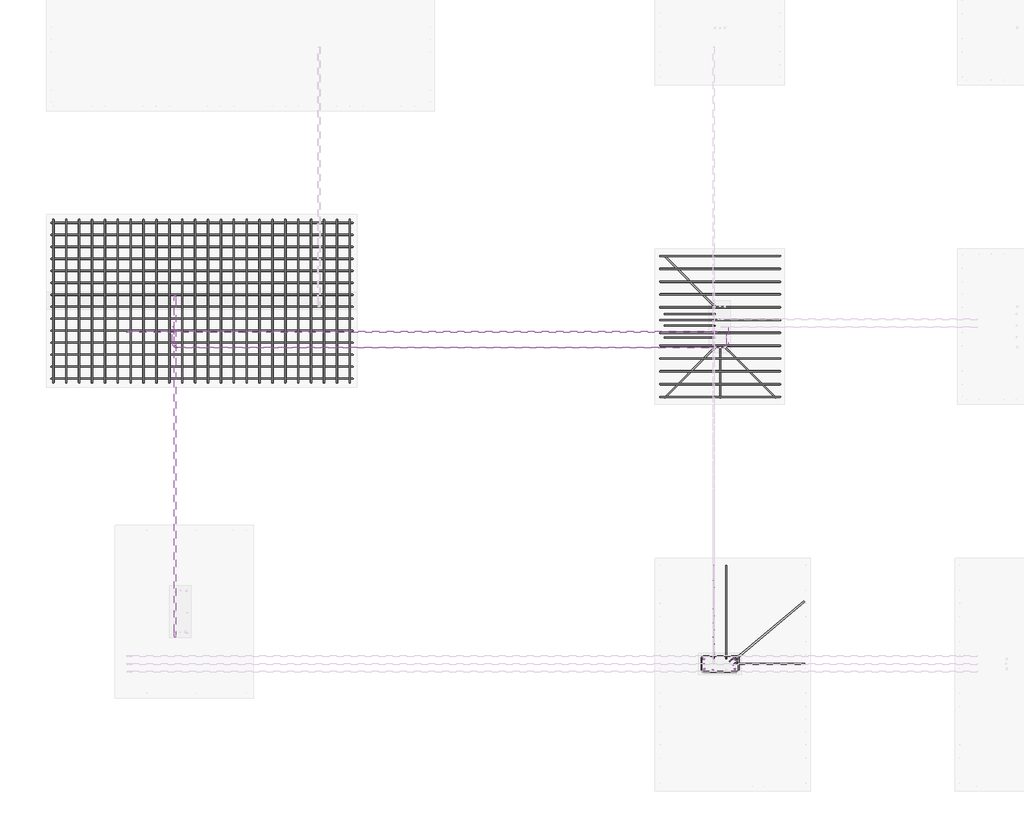
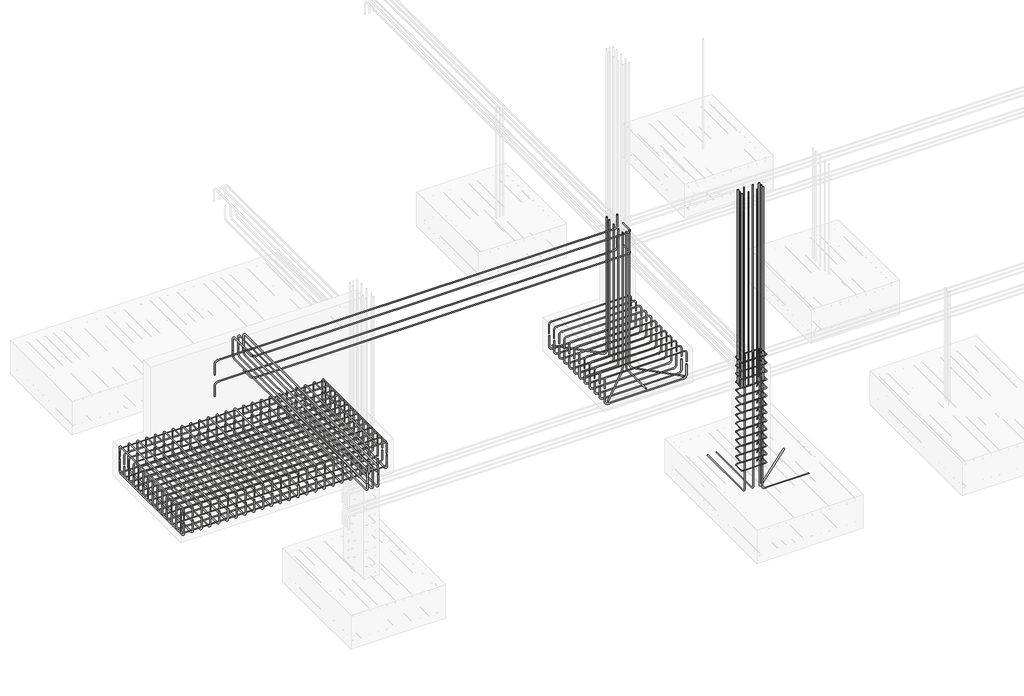
# One storey, part 3 of 18: 27 reinforcing bars.
"""IFC4 building model written with IfcOpenShell, lengths in millimetres."""

from ifc_helpers import new_model, si_unit, point, frame, origin, place, context, project, spatial, polyline, circle_curve, trimmed, segment, composite_curve, source, transform, mapped, element, save
from ifc_brep_helpers import swept_disk

model = new_model("IFC4")

# Units and contexts
model_context = context("Model", 3, world=origin())
ifc_project = project(units=[si_unit("LENGTHUNIT", "METRE", prefix="MILLI")], contexts=[model_context])

# Site, building, storey
site = spatial("IfcSite", under=ifc_project)
building = spatial("IfcBuilding", under=site)
storey = spatial("IfcBuildingStorey", under=building, Elevation=-2000.0)

# Reinforcing bars
placement = place(None, origin())
reinforcing_bar_shape = source(origin(), model_context, "Body", "SolidModel", [
    swept_disk(composite_curve([segment(polyline([(-16391.7335738, -415.3521146, -2300.0), (-16391.7335738, -415.3521146, -2486.6)]), True, "CONTINUOUS"), segment(trimmed(circle_curve(frame((-16391.7335738, -470.8021146, -2486.6), z_axis=(-1.0, 0.0, 0.0), x_axis=(0.0, 55.44999999999999, 0.0)), 55.45), [point((-16391.7335738, -415.3521146, -2486.6))], [point((-16391.7335738, -470.8021146, -2542.05))], True, "CARTESIAN"), True, "CONTINUOUS"), segment(polyline([(-16391.7335738, -470.8021146, -2542.05), (-16391.7335738, -2244.0021146, -2542.05)]), True, "CONTINUOUS"), segment(trimmed(circle_curve(frame((-16391.7335738, -2244.0021146, -2486.6), z_axis=(-1.0, 0.0, 0.0), x_axis=(0.0, 0.0, -55.45000000000027)), 55.45), [point((-16391.7335738, -2244.0021146, -2542.05))], [point((-16391.7335738, -2299.4521146, -2486.6))], True, "CARTESIAN"), True, "CONTINUOUS"), segment(polyline([(-16391.7335738, -2299.4521146, -2486.6), (-16391.7335738, -2299.4521146, -2300.0)]), True, "CONTINUOUS")], self_intersect=False), 7.95),
])
element("IfcReinforcingBar", 1, at=placement, inside=storey, context=model_context, shape_type="MappedRepresentation", body=[
    mapped(reinforcing_bar_shape, transform((0.0, 0.0, 0.0), x_axis=(1.0, 0.0, 0.0), y_axis=(0.0, 1.0, 0.0), z_axis=(0.0, 0.0, 1.0))),
    mapped(reinforcing_bar_shape, transform((149.246773, 0.0, 0.0), x_axis=(1.0, 0.0, 0.0), y_axis=(0.0, 1.0, 0.0), z_axis=(0.0, 0.0, 1.0))),
    mapped(reinforcing_bar_shape, transform((298.4935461, 0.0, 0.0), x_axis=(1.0, 0.0, 0.0), y_axis=(0.0, 1.0, 0.0), z_axis=(0.0, 0.0, 1.0))),
    mapped(reinforcing_bar_shape, transform((447.7403191, 0.0, 0.0), x_axis=(1.0, 0.0, 0.0), y_axis=(0.0, 1.0, 0.0), z_axis=(0.0, 0.0, 1.0))),
    mapped(reinforcing_bar_shape, transform((596.9870921, 0.0, 0.0), x_axis=(1.0, 0.0, 0.0), y_axis=(0.0, 1.0, 0.0), z_axis=(0.0, 0.0, 1.0))),
    mapped(reinforcing_bar_shape, transform((746.2338651, 0.0, 0.0), x_axis=(1.0, 0.0, 0.0), y_axis=(0.0, 1.0, 0.0), z_axis=(0.0, 0.0, 1.0))),
    mapped(reinforcing_bar_shape, transform((895.4806382, 0.0, 0.0), x_axis=(1.0, 0.0, 0.0), y_axis=(0.0, 1.0, 0.0), z_axis=(0.0, 0.0, 1.0))),
    mapped(reinforcing_bar_shape, transform((1044.7274112, 0.0, 0.0), x_axis=(1.0, 0.0, 0.0), y_axis=(0.0, 1.0, 0.0), z_axis=(0.0, 0.0, 1.0))),
    mapped(reinforcing_bar_shape, transform((1193.9741842, 0.0, 0.0), x_axis=(1.0, 0.0, 0.0), y_axis=(0.0, 1.0, 0.0), z_axis=(0.0, 0.0, 1.0))),
    mapped(reinforcing_bar_shape, transform((1343.2209572, 0.0, 0.0), x_axis=(1.0, 0.0, 0.0), y_axis=(0.0, 1.0, 0.0), z_axis=(0.0, 0.0, 1.0))),
    mapped(reinforcing_bar_shape, transform((1492.4677303, 0.0, 0.0), x_axis=(1.0, 0.0, 0.0), y_axis=(0.0, 1.0, 0.0), z_axis=(0.0, 0.0, 1.0))),
    mapped(reinforcing_bar_shape, transform((1641.7145033, 0.0, 0.0), x_axis=(1.0, 0.0, 0.0), y_axis=(0.0, 1.0, 0.0), z_axis=(0.0, 0.0, 1.0))),
    mapped(reinforcing_bar_shape, transform((1790.9612763, 0.0, 0.0), x_axis=(1.0, 0.0, 0.0), y_axis=(0.0, 1.0, 0.0), z_axis=(0.0, 0.0, 1.0))),
    mapped(reinforcing_bar_shape, transform((1940.2080494, 0.0, 0.0), x_axis=(1.0, 0.0, 0.0), y_axis=(0.0, 1.0, 0.0), z_axis=(0.0, 0.0, 1.0))),
    mapped(reinforcing_bar_shape, transform((2089.4548224, 0.0, 0.0), x_axis=(1.0, 0.0, 0.0), y_axis=(0.0, 1.0, 0.0), z_axis=(0.0, 0.0, 1.0))),
    mapped(reinforcing_bar_shape, transform((2238.7015954, 0.0, 0.0), x_axis=(1.0, 0.0, 0.0), y_axis=(0.0, 1.0, 0.0), z_axis=(0.0, 0.0, 1.0))),
    mapped(reinforcing_bar_shape, transform((2387.9483684, 0.0, 0.0), x_axis=(1.0, 0.0, 0.0), y_axis=(0.0, 1.0, 0.0), z_axis=(0.0, 0.0, 1.0))),
    mapped(reinforcing_bar_shape, transform((2537.1951415, 0.0, 0.0), x_axis=(1.0, 0.0, 0.0), y_axis=(0.0, 1.0, 0.0), z_axis=(0.0, 0.0, 1.0))),
    mapped(reinforcing_bar_shape, transform((2686.4419145, 0.0, 0.0), x_axis=(1.0, 0.0, 0.0), y_axis=(0.0, 1.0, 0.0), z_axis=(0.0, 0.0, 1.0))),
    mapped(reinforcing_bar_shape, transform((2835.6886875, 0.0, 0.0), x_axis=(1.0, 0.0, 0.0), y_axis=(0.0, 1.0, 0.0), z_axis=(0.0, 0.0, 1.0))),
    mapped(reinforcing_bar_shape, transform((2984.9354605, 0.0, 0.0), x_axis=(1.0, 0.0, 0.0), y_axis=(0.0, 1.0, 0.0), z_axis=(0.0, 0.0, 1.0))),
    mapped(reinforcing_bar_shape, transform((3134.1822336, 0.0, 0.0), x_axis=(1.0, 0.0, 0.0), y_axis=(0.0, 1.0, 0.0), z_axis=(0.0, 0.0, 1.0))),
    mapped(reinforcing_bar_shape, transform((3283.4290066, 0.0, 0.0), x_axis=(1.0, 0.0, 0.0), y_axis=(0.0, 1.0, 0.0), z_axis=(0.0, 0.0, 1.0))),
    mapped(reinforcing_bar_shape, transform((3432.6757796, 0.0, 0.0), x_axis=(1.0, 0.0, 0.0), y_axis=(0.0, 1.0, 0.0), z_axis=(0.0, 0.0, 1.0))),
])
reinforcing_bar_2_shape = source(origin(), model_context, "Body", "SolidModel", [
    swept_disk(composite_curve([segment(polyline([(-16391.7335738, -2301.4021146, -2250.0), (-16391.7335738, -2301.4021146, -2102.0)]), True, "CONTINUOUS"), segment(trimmed(circle_curve(frame((-16391.7335738, -2255.4021146, -2102.0), z_axis=(-1.0, 0.0, 0.0), x_axis=(0.0, -46.0, 0.0)), 46.0), [point((-16391.7335738, -2301.4021146, -2102.0))], [point((-16391.7335738, -2255.4021146, -2056.0))], True, "CARTESIAN"), True, "CONTINUOUS"), segment(polyline([(-16391.7335738, -2255.4021146, -2056.0), (-16391.7335738, -459.4021146, -2056.0)]), True, "CONTINUOUS"), segment(trimmed(circle_curve(frame((-16391.7335738, -459.4021146, -2102.0), z_axis=(-1.0, 0.0, 0.0), x_axis=(0.0, 0.0, 46.0)), 46.0), [point((-16391.7335738, -459.4021146, -2056.0))], [point((-16391.7335738, -413.4021146, -2102.0))], True, "CARTESIAN"), True, "CONTINUOUS"), segment(polyline([(-16391.7335738, -413.4021146, -2102.0), (-16391.7335738, -413.4021146, -2250.0)]), True, "CONTINUOUS")], self_intersect=False), 6.0),
])
element("IfcReinforcingBar", 2, at=placement, inside=storey, context=model_context, shape_type="MappedRepresentation", body=[
    mapped(reinforcing_bar_2_shape, transform((0.0, 0.0, 0.0), x_axis=(1.0, 0.0, 0.0), y_axis=(0.0, 1.0, 0.0), z_axis=(0.0, 0.0, 1.0))),
    mapped(reinforcing_bar_2_shape, transform((149.246773, 0.0, 0.0), x_axis=(1.0, 0.0, 0.0), y_axis=(0.0, 1.0, 0.0), z_axis=(0.0, 0.0, 1.0))),
    mapped(reinforcing_bar_2_shape, transform((298.4935461, 0.0, 0.0), x_axis=(1.0, 0.0, 0.0), y_axis=(0.0, 1.0, 0.0), z_axis=(0.0, 0.0, 1.0))),
    mapped(reinforcing_bar_2_shape, transform((447.7403191, 0.0, 0.0), x_axis=(1.0, 0.0, 0.0), y_axis=(0.0, 1.0, 0.0), z_axis=(0.0, 0.0, 1.0))),
    mapped(reinforcing_bar_2_shape, transform((596.9870921, 0.0, 0.0), x_axis=(1.0, 0.0, 0.0), y_axis=(0.0, 1.0, 0.0), z_axis=(0.0, 0.0, 1.0))),
    mapped(reinforcing_bar_2_shape, transform((746.2338651, 0.0, 0.0), x_axis=(1.0, 0.0, 0.0), y_axis=(0.0, 1.0, 0.0), z_axis=(0.0, 0.0, 1.0))),
    mapped(reinforcing_bar_2_shape, transform((895.4806382, 0.0, 0.0), x_axis=(1.0, 0.0, 0.0), y_axis=(0.0, 1.0, 0.0), z_axis=(0.0, 0.0, 1.0))),
    mapped(reinforcing_bar_2_shape, transform((1044.7274112, 0.0, 0.0), x_axis=(1.0, 0.0, 0.0), y_axis=(0.0, 1.0, 0.0), z_axis=(0.0, 0.0, 1.0))),
    mapped(reinforcing_bar_2_shape, transform((1193.9741842, 0.0, 0.0), x_axis=(1.0, 0.0, 0.0), y_axis=(0.0, 1.0, 0.0), z_axis=(0.0, 0.0, 1.0))),
    mapped(reinforcing_bar_2_shape, transform((1343.2209572, 0.0, 0.0), x_axis=(1.0, 0.0, 0.0), y_axis=(0.0, 1.0, 0.0), z_axis=(0.0, 0.0, 1.0))),
    mapped(reinforcing_bar_2_shape, transform((1492.4677303, 0.0, 0.0), x_axis=(1.0, 0.0, 0.0), y_axis=(0.0, 1.0, 0.0), z_axis=(0.0, 0.0, 1.0))),
    mapped(reinforcing_bar_2_shape, transform((1641.7145033, 0.0, 0.0), x_axis=(1.0, 0.0, 0.0), y_axis=(0.0, 1.0, 0.0), z_axis=(0.0, 0.0, 1.0))),
    mapped(reinforcing_bar_2_shape, transform((1790.9612763, 0.0, 0.0), x_axis=(1.0, 0.0, 0.0), y_axis=(0.0, 1.0, 0.0), z_axis=(0.0, 0.0, 1.0))),
    mapped(reinforcing_bar_2_shape, transform((1940.2080494, 0.0, 0.0), x_axis=(1.0, 0.0, 0.0), y_axis=(0.0, 1.0, 0.0), z_axis=(0.0, 0.0, 1.0))),
    mapped(reinforcing_bar_2_shape, transform((2089.4548224, 0.0, 0.0), x_axis=(1.0, 0.0, 0.0), y_axis=(0.0, 1.0, 0.0), z_axis=(0.0, 0.0, 1.0))),
    mapped(reinforcing_bar_2_shape, transform((2238.7015954, 0.0, 0.0), x_axis=(1.0, 0.0, 0.0), y_axis=(0.0, 1.0, 0.0), z_axis=(0.0, 0.0, 1.0))),
    mapped(reinforcing_bar_2_shape, transform((2387.9483684, 0.0, 0.0), x_axis=(1.0, 0.0, 0.0), y_axis=(0.0, 1.0, 0.0), z_axis=(0.0, 0.0, 1.0))),
    mapped(reinforcing_bar_2_shape, transform((2537.1951415, 0.0, 0.0), x_axis=(1.0, 0.0, 0.0), y_axis=(0.0, 1.0, 0.0), z_axis=(0.0, 0.0, 1.0))),
    mapped(reinforcing_bar_2_shape, transform((2686.4419145, 0.0, 0.0), x_axis=(1.0, 0.0, 0.0), y_axis=(0.0, 1.0, 0.0), z_axis=(0.0, 0.0, 1.0))),
    mapped(reinforcing_bar_2_shape, transform((2835.6886875, 0.0, 0.0), x_axis=(1.0, 0.0, 0.0), y_axis=(0.0, 1.0, 0.0), z_axis=(0.0, 0.0, 1.0))),
    mapped(reinforcing_bar_2_shape, transform((2984.9354605, 0.0, 0.0), x_axis=(1.0, 0.0, 0.0), y_axis=(0.0, 1.0, 0.0), z_axis=(0.0, 0.0, 1.0))),
    mapped(reinforcing_bar_2_shape, transform((3134.1822336, 0.0, 0.0), x_axis=(1.0, 0.0, 0.0), y_axis=(0.0, 1.0, 0.0), z_axis=(0.0, 0.0, 1.0))),
    mapped(reinforcing_bar_2_shape, transform((3283.4290066, 0.0, 0.0), x_axis=(1.0, 0.0, 0.0), y_axis=(0.0, 1.0, 0.0), z_axis=(0.0, 0.0, 1.0))),
    mapped(reinforcing_bar_2_shape, transform((3432.6757796, 0.0, 0.0), x_axis=(1.0, 0.0, 0.0), y_axis=(0.0, 1.0, 0.0), z_axis=(0.0, 0.0, 1.0))),
])
reinforcing_bar_3_shape = source(origin(), model_context, "Body", "SolidModel", [
    swept_disk(composite_curve([segment(polyline([(-16414.6290491, -2255.2213318, -2322.6684255), (-16414.6290491, -2255.2213318, -2470.6684255)]), True, "CONTINUOUS"), segment(trimmed(circle_curve(frame((-16368.6290491, -2255.2213318, -2470.6684255), z_axis=(0.0, -1.0, 0.0), x_axis=(-46.0, 0.0, 0.0)), 46.0), [point((-16414.6290491, -2255.2213318, -2470.6684255))], [point((-16368.6290491, -2255.2213318, -2516.6684255))], True, "CARTESIAN"), True, "CONTINUOUS"), segment(polyline([(-16368.6290491, -2255.2213318, -2516.6684255), (-12972.6290491, -2255.2213318, -2516.6684255)]), True, "CONTINUOUS"), segment(trimmed(circle_curve(frame((-12972.6290491, -2255.2213318, -2470.6684255), z_axis=(0.0, -1.0, 0.0), x_axis=(0.0, 0.0, -46.0)), 46.0), [point((-12972.6290491, -2255.2213318, -2516.6684255))], [point((-12926.6290491, -2255.2213318, -2470.6684255))], True, "CARTESIAN"), True, "CONTINUOUS"), segment(polyline([(-12926.6290491, -2255.2213318, -2470.6684255), (-12926.6290491, -2255.2213318, -2322.6684255)]), True, "CONTINUOUS")], self_intersect=False), 6.0),
])
element("IfcReinforcingBar", 3, at=placement, inside=storey, context=model_context, shape_type="MappedRepresentation", body=[
    mapped(reinforcing_bar_3_shape, transform((0.0, 0.0, 0.0), x_axis=(1.0, 0.0, 0.0), y_axis=(0.0, 1.0, 0.0), z_axis=(0.0, 0.0, 1.0))),
    mapped(reinforcing_bar_3_shape, transform((0.0, 138.7553125, 0.0), x_axis=(1.0, 0.0, 0.0), y_axis=(0.0, 1.0, 0.0), z_axis=(0.0, 0.0, 1.0))),
    mapped(reinforcing_bar_3_shape, transform((0.0, 277.510625, 0.0), x_axis=(1.0, 0.0, 0.0), y_axis=(0.0, 1.0, 0.0), z_axis=(0.0, 0.0, 1.0))),
    mapped(reinforcing_bar_3_shape, transform((0.0, 416.2659375, 0.0), x_axis=(1.0, 0.0, 0.0), y_axis=(0.0, 1.0, 0.0), z_axis=(0.0, 0.0, 1.0))),
    mapped(reinforcing_bar_3_shape, transform((0.0, 555.02125, 0.0), x_axis=(1.0, 0.0, 0.0), y_axis=(0.0, 1.0, 0.0), z_axis=(0.0, 0.0, 1.0))),
    mapped(reinforcing_bar_3_shape, transform((0.0, 693.7765624, 0.0), x_axis=(1.0, 0.0, 0.0), y_axis=(0.0, 1.0, 0.0), z_axis=(0.0, 0.0, 1.0))),
    mapped(reinforcing_bar_3_shape, transform((0.0, 832.5318749, 0.0), x_axis=(1.0, 0.0, 0.0), y_axis=(0.0, 1.0, 0.0), z_axis=(0.0, 0.0, 1.0))),
    mapped(reinforcing_bar_3_shape, transform((0.0, 971.2871874, 0.0), x_axis=(1.0, 0.0, 0.0), y_axis=(0.0, 1.0, 0.0), z_axis=(0.0, 0.0, 1.0))),
    mapped(reinforcing_bar_3_shape, transform((0.0, 1110.0424999, 0.0), x_axis=(1.0, 0.0, 0.0), y_axis=(0.0, 1.0, 0.0), z_axis=(0.0, 0.0, 1.0))),
    mapped(reinforcing_bar_3_shape, transform((0.0, 1248.7978124, 0.0), x_axis=(1.0, 0.0, 0.0), y_axis=(0.0, 1.0, 0.0), z_axis=(0.0, 0.0, 1.0))),
    mapped(reinforcing_bar_3_shape, transform((0.0, 1387.5531249, 0.0), x_axis=(1.0, 0.0, 0.0), y_axis=(0.0, 1.0, 0.0), z_axis=(0.0, 0.0, 1.0))),
    mapped(reinforcing_bar_3_shape, transform((0.0, 1526.3084374, 0.0), x_axis=(1.0, 0.0, 0.0), y_axis=(0.0, 1.0, 0.0), z_axis=(0.0, 0.0, 1.0))),
    mapped(reinforcing_bar_3_shape, transform((0.0, 1665.0637499, 0.0), x_axis=(1.0, 0.0, 0.0), y_axis=(0.0, 1.0, 0.0), z_axis=(0.0, 0.0, 1.0))),
    mapped(reinforcing_bar_3_shape, transform((0.0, 1803.8190623, 0.0), x_axis=(1.0, 0.0, 0.0), y_axis=(0.0, 1.0, 0.0), z_axis=(0.0, 0.0, 1.0))),
])
reinforcing_bar_4_shape = source(origin(), model_context, "Body", "SolidModel", [
    swept_disk(composite_curve([segment(polyline([(-16414.6290491, -449.4790976, -2276.6677805), (-16414.6290491, -449.4790976, -2128.6677805)]), True, "CONTINUOUS"), segment(trimmed(circle_curve(frame((-16368.6290491, -449.4790976, -2128.6677805), z_axis=(0.0, 1.0, 0.0), x_axis=(-46.0, 0.0, 0.0)), 46.0), [point((-16414.6290491, -449.4790976, -2128.6677805))], [point((-16368.6290491, -449.4790976, -2082.6677805))], True, "CARTESIAN"), True, "CONTINUOUS"), segment(polyline([(-16368.6290491, -449.4790976, -2082.6677805), (-12972.6290491, -449.4790976, -2082.6677805)]), True, "CONTINUOUS"), segment(trimmed(circle_curve(frame((-12972.6290491, -449.4790976, -2128.6677805), z_axis=(0.0, 1.0, 0.0), x_axis=(0.0, 0.0, 46.0)), 46.0), [point((-12972.6290491, -449.4790976, -2082.6677805))], [point((-12926.6290491, -449.4790976, -2128.6677805))], True, "CARTESIAN"), True, "CONTINUOUS"), segment(polyline([(-12926.6290491, -449.4790976, -2128.6677805), (-12926.6290491, -449.4790976, -2276.6677805)]), True, "CONTINUOUS")], self_intersect=False), 6.0),
])
element("IfcReinforcingBar", 4, at=placement, inside=storey, context=model_context, shape_type="MappedRepresentation", body=[
    mapped(reinforcing_bar_4_shape, transform((0.0, 0.0, 0.0), x_axis=(1.0, 0.0, 0.0), y_axis=(0.0, 1.0, 0.0), z_axis=(0.0, 0.0, 1.0))),
    mapped(reinforcing_bar_4_shape, transform((0.0, -138.9032488, 0.0), x_axis=(1.0, 0.0, 0.0), y_axis=(0.0, 1.0, 0.0), z_axis=(0.0, 0.0, 1.0))),
    mapped(reinforcing_bar_4_shape, transform((0.0, -277.8064976, 0.0), x_axis=(1.0, 0.0, 0.0), y_axis=(0.0, 1.0, 0.0), z_axis=(0.0, 0.0, 1.0))),
    mapped(reinforcing_bar_4_shape, transform((0.0, -416.7097463, 0.0), x_axis=(1.0, 0.0, 0.0), y_axis=(0.0, 1.0, 0.0), z_axis=(0.0, 0.0, 1.0))),
    mapped(reinforcing_bar_4_shape, transform((0.0, -555.6129951, 0.0), x_axis=(1.0, 0.0, 0.0), y_axis=(0.0, 1.0, 0.0), z_axis=(0.0, 0.0, 1.0))),
    mapped(reinforcing_bar_4_shape, transform((0.0, -694.5162439, 0.0), x_axis=(1.0, 0.0, 0.0), y_axis=(0.0, 1.0, 0.0), z_axis=(0.0, 0.0, 1.0))),
    mapped(reinforcing_bar_4_shape, transform((0.0, -833.4194927, 0.0), x_axis=(1.0, 0.0, 0.0), y_axis=(0.0, 1.0, 0.0), z_axis=(0.0, 0.0, 1.0))),
    mapped(reinforcing_bar_4_shape, transform((0.0, -972.3227415, 0.0), x_axis=(1.0, 0.0, 0.0), y_axis=(0.0, 1.0, 0.0), z_axis=(0.0, 0.0, 1.0))),
    mapped(reinforcing_bar_4_shape, transform((0.0, -1111.2259903, 0.0), x_axis=(1.0, 0.0, 0.0), y_axis=(0.0, 1.0, 0.0), z_axis=(0.0, 0.0, 1.0))),
    mapped(reinforcing_bar_4_shape, transform((0.0, -1250.129239, 0.0), x_axis=(1.0, 0.0, 0.0), y_axis=(0.0, 1.0, 0.0), z_axis=(0.0, 0.0, 1.0))),
    mapped(reinforcing_bar_4_shape, transform((0.0, -1389.0324878, 0.0), x_axis=(1.0, 0.0, 0.0), y_axis=(0.0, 1.0, 0.0), z_axis=(0.0, 0.0, 1.0))),
    mapped(reinforcing_bar_4_shape, transform((0.0, -1527.9357366, 0.0), x_axis=(1.0, 0.0, 0.0), y_axis=(0.0, 1.0, 0.0), z_axis=(0.0, 0.0, 1.0))),
    mapped(reinforcing_bar_4_shape, transform((0.0, -1666.8389854, 0.0), x_axis=(1.0, 0.0, 0.0), y_axis=(0.0, 1.0, 0.0), z_axis=(0.0, 0.0, 1.0))),
    mapped(reinforcing_bar_4_shape, transform((0.0, -1805.7422342, 0.0), x_axis=(1.0, 0.0, 0.0), y_axis=(0.0, 1.0, 0.0), z_axis=(0.0, 0.0, 1.0))),
])
reinforcing_bar_5_shape = source(origin(), model_context, "Body", "SolidModel", [
    swept_disk(composite_curve([segment(polyline([(-7978.5399692, -834.8555128, -2300.0), (-7978.5399692, -834.8555128, -2486.6)]), True, "CONTINUOUS"), segment(trimmed(circle_curve(frame((-8033.9899692, -834.8555128, -2486.6), z_axis=(0.0, 1.0, 0.0), x_axis=(55.44999999999982, 0.0, 0.0)), 55.45), [point((-7978.5399692, -834.8555128, -2486.6))], [point((-8033.9899692, -834.8555128, -2542.05))], True, "CARTESIAN"), True, "CONTINUOUS"), segment(polyline([(-8033.9899692, -834.8555128, -2542.05), (-9307.1899692, -834.8555128, -2542.05)]), True, "CONTINUOUS"), segment(trimmed(circle_curve(frame((-9307.1899692, -834.8555128, -2486.6), z_axis=(0.0, 1.0, 0.0), x_axis=(0.0, 0.0, -55.45000000000027)), 55.45), [point((-9307.1899692, -834.8555128, -2542.05))], [point((-9362.6399692, -834.8555128, -2486.6))], True, "CARTESIAN"), True, "CONTINUOUS"), segment(polyline([(-9362.6399692, -834.8555128, -2486.6), (-9362.6399692, -834.8555128, -2300.0)]), True, "CONTINUOUS")], self_intersect=False), 7.95),
])
element("IfcReinforcingBar", 5, at=placement, inside=storey, context=model_context, shape_type="MappedRepresentation", body=[
    mapped(reinforcing_bar_5_shape, transform((0.0, 0.0, 0.0), x_axis=(1.0, 0.0, 0.0), y_axis=(0.0, 1.0, 0.0), z_axis=(0.0, 0.0, 1.0))),
    mapped(reinforcing_bar_5_shape, transform((0.0, -148.4250709, 0.0), x_axis=(1.0, 0.0, 0.0), y_axis=(0.0, 1.0, 0.0), z_axis=(0.0, 0.0, 1.0))),
    mapped(reinforcing_bar_5_shape, transform((0.0, -296.8501418, 0.0), x_axis=(1.0, 0.0, 0.0), y_axis=(0.0, 1.0, 0.0), z_axis=(0.0, 0.0, 1.0))),
    mapped(reinforcing_bar_5_shape, transform((0.0, -445.2752126, 0.0), x_axis=(1.0, 0.0, 0.0), y_axis=(0.0, 1.0, 0.0), z_axis=(0.0, 0.0, 1.0))),
    mapped(reinforcing_bar_5_shape, transform((0.0, -593.7002835, 0.0), x_axis=(1.0, 0.0, 0.0), y_axis=(0.0, 1.0, 0.0), z_axis=(0.0, 0.0, 1.0))),
    mapped(reinforcing_bar_5_shape, transform((0.0, -742.1253544, 0.0), x_axis=(1.0, 0.0, 0.0), y_axis=(0.0, 1.0, 0.0), z_axis=(0.0, 0.0, 1.0))),
    mapped(reinforcing_bar_5_shape, transform((0.0, -890.5504253, 0.0), x_axis=(1.0, 0.0, 0.0), y_axis=(0.0, 1.0, 0.0), z_axis=(0.0, 0.0, 1.0))),
    mapped(reinforcing_bar_5_shape, transform((0.0, -1038.9754961, 0.0), x_axis=(1.0, 0.0, 0.0), y_axis=(0.0, 1.0, 0.0), z_axis=(0.0, 0.0, 1.0))),
    mapped(reinforcing_bar_5_shape, transform((0.0, -1187.400567, 0.0), x_axis=(1.0, 0.0, 0.0), y_axis=(0.0, 1.0, 0.0), z_axis=(0.0, 0.0, 1.0))),
    mapped(reinforcing_bar_5_shape, transform((0.0, -1335.8256379, 0.0), x_axis=(1.0, 0.0, 0.0), y_axis=(0.0, 1.0, 0.0), z_axis=(0.0, 0.0, 1.0))),
    mapped(reinforcing_bar_5_shape, transform((0.0, -1484.2507088, 0.0), x_axis=(1.0, 0.0, 0.0), y_axis=(0.0, 1.0, 0.0), z_axis=(0.0, 0.0, 1.0))),
    mapped(reinforcing_bar_5_shape, transform((0.0, -1632.6757796, 0.0), x_axis=(1.0, 0.0, 0.0), y_axis=(0.0, 1.0, 0.0), z_axis=(0.0, 0.0, 1.0))),
])
reinforcing_bar_6_shape = source(origin(), model_context, "Body", "SolidModel", [
    swept_disk(composite_curve([segment(polyline([(-9364.5899692, -834.8555128, -2250.0), (-9364.5899692, -834.8555128, -2102.0)]), True, "CONTINUOUS"), segment(trimmed(circle_curve(frame((-9318.5899692, -834.8555128, -2102.0), z_axis=(0.0, 1.0, 0.0), x_axis=(-46.0, 0.0, 0.0)), 46.0), [point((-9364.5899692, -834.8555128, -2102.0))], [point((-9318.5899692, -834.8555128, -2056.0))], True, "CARTESIAN"), True, "CONTINUOUS"), segment(polyline([(-9318.5899692, -834.8555128, -2056.0), (-8022.5899692, -834.8555128, -2056.0)]), True, "CONTINUOUS"), segment(trimmed(circle_curve(frame((-8022.5899692, -834.8555128, -2102.0), z_axis=(0.0, 1.0, 0.0), x_axis=(0.0, 0.0, 46.0)), 46.0), [point((-8022.5899692, -834.8555128, -2056.0))], [point((-7976.5899692, -834.8555128, -2102.0))], True, "CARTESIAN"), True, "CONTINUOUS"), segment(polyline([(-7976.5899692, -834.8555128, -2102.0), (-7976.5899692, -834.8555128, -2250.0)]), True, "CONTINUOUS")], self_intersect=False), 6.0),
])
element("IfcReinforcingBar", 6, at=placement, inside=storey, context=model_context, shape_type="MappedRepresentation", body=[
    mapped(reinforcing_bar_6_shape, transform((0.0, 0.0, 0.0), x_axis=(1.0, 0.0, 0.0), y_axis=(0.0, 1.0, 0.0), z_axis=(0.0, 0.0, 1.0))),
    mapped(reinforcing_bar_6_shape, transform((0.0, -148.4250709, 0.0), x_axis=(1.0, 0.0, 0.0), y_axis=(0.0, 1.0, 0.0), z_axis=(0.0, 0.0, 1.0))),
    mapped(reinforcing_bar_6_shape, transform((0.0, -296.8501418, 0.0), x_axis=(1.0, 0.0, 0.0), y_axis=(0.0, 1.0, 0.0), z_axis=(0.0, 0.0, 1.0))),
    mapped(reinforcing_bar_6_shape, transform((0.0, -445.2752126, 0.0), x_axis=(1.0, 0.0, 0.0), y_axis=(0.0, 1.0, 0.0), z_axis=(0.0, 0.0, 1.0))),
    mapped(reinforcing_bar_6_shape, transform((0.0, -593.7002835, 0.0), x_axis=(1.0, 0.0, 0.0), y_axis=(0.0, 1.0, 0.0), z_axis=(0.0, 0.0, 1.0))),
    mapped(reinforcing_bar_6_shape, transform((0.0, -742.1253544, 0.0), x_axis=(1.0, 0.0, 0.0), y_axis=(0.0, 1.0, 0.0), z_axis=(0.0, 0.0, 1.0))),
    mapped(reinforcing_bar_6_shape, transform((0.0, -890.5504253, 0.0), x_axis=(1.0, 0.0, 0.0), y_axis=(0.0, 1.0, 0.0), z_axis=(0.0, 0.0, 1.0))),
    mapped(reinforcing_bar_6_shape, transform((0.0, -1038.9754961, 0.0), x_axis=(1.0, 0.0, 0.0), y_axis=(0.0, 1.0, 0.0), z_axis=(0.0, 0.0, 1.0))),
    mapped(reinforcing_bar_6_shape, transform((0.0, -1187.400567, 0.0), x_axis=(1.0, 0.0, 0.0), y_axis=(0.0, 1.0, 0.0), z_axis=(0.0, 0.0, 1.0))),
    mapped(reinforcing_bar_6_shape, transform((0.0, -1335.8256379, 0.0), x_axis=(1.0, 0.0, 0.0), y_axis=(0.0, 1.0, 0.0), z_axis=(0.0, 0.0, 1.0))),
    mapped(reinforcing_bar_6_shape, transform((0.0, -1484.2507088, 0.0), x_axis=(1.0, 0.0, 0.0), y_axis=(0.0, 1.0, 0.0), z_axis=(0.0, 0.0, 1.0))),
    mapped(reinforcing_bar_6_shape, transform((0.0, -1632.6757796, 0.0), x_axis=(1.0, 0.0, 0.0), y_axis=(0.0, 1.0, 0.0), z_axis=(0.0, 0.0, 1.0))),
])
reinforcing_bar_7_shape = source(origin(), model_context, "Body", "SolidModel", [
    swept_disk(composite_curve([segment(polyline([(-8560.4315175, -5535.5091206, -34.0), (-8504.0960659, -5479.1736689, -34.0)]), True, "CONTINUOUS"), segment(trimmed(circle_curve(frame((-8483.5899692, -5499.6797656, -34.0), z_axis=(0.0, 0.0, -1.0), x_axis=(-20.506096699999034, 20.506096699999944, 0.0)), 29.0), [point((-8504.0960659, -5479.1736689, -34.0))], [point((-8454.5899692, -5499.6797656, -34.0))], True, "CARTESIAN"), True, "CONTINUOUS"), segment(polyline([(-8454.5899692, -5499.6797656, -34.0), (-8454.5899692, -5623.6797656, -34.0)]), True, "CONTINUOUS"), segment(trimmed(circle_curve(frame((-8483.5899692, -5623.6797656, -34.0), z_axis=(0.0, 0.0, -1.0), x_axis=(29.0, 0.0, 0.0)), 29.0), [point((-8454.5899692, -5623.6797656, -34.0))], [point((-8483.5899692, -5652.6797656, -34.0))], True, "CARTESIAN"), True, "CONTINUOUS"), segment(polyline([(-8483.5899692, -5652.6797656, -34.0), (-8857.5899692, -5652.6797656, -34.0)]), True, "CONTINUOUS"), segment(trimmed(circle_curve(frame((-8857.5899692, -5623.707741, -32.7265044), z_axis=(0.0, 0.043913640913297095, -0.9990353307775146), x_axis=(0.0, -28.972024599999713, -1.2734955999999968)), 29.0), [point((-8857.5899692, -5652.6797656, -34.0))], [point((-8886.5899692, -5623.707741, -32.7265044))], True, "CARTESIAN"), True, "CONTINUOUS"), segment(polyline([(-8886.5899692, -5623.707741, -32.7265044), (-8886.5899692, -5499.6517902, -27.2734956)]), True, "CONTINUOUS"), segment(trimmed(circle_curve(frame((-8857.5899692, -5499.6517902, -27.2734956), z_axis=(0.0, 0.043913640913297095, -0.9990353307775146), x_axis=(-29.0, 0.0, 0.0)), 29.0), [point((-8886.5899692, -5499.6517902, -27.2734956))], [point((-8857.5899692, -5470.6797656, -26.0))], True, "CARTESIAN"), True, "CONTINUOUS"), segment(polyline([(-8857.5899692, -5470.6797656, -26.0), (-8483.5899692, -5470.6797656, -26.0)]), True, "CONTINUOUS"), segment(trimmed(circle_curve(frame((-8483.5899692, -5499.6797656, -26.0), z_axis=(0.0, 0.0, -1.0), x_axis=(0.0, 29.0, 0.0)), 29.0), [point((-8483.5899692, -5470.6797656, -26.0))], [point((-8463.0838726, -5520.1858622, -26.0))], True, "CARTESIAN"), True, "CONTINUOUS"), segment(polyline([(-8463.0838726, -5520.1858622, -26.0), (-8519.4193242, -5576.5213139, -26.0)]), True, "CONTINUOUS")], self_intersect=False), 4.0),
])
element("IfcReinforcingBar", 7, at=placement, inside=storey, context=model_context, shape_type="MappedRepresentation", body=[
    mapped(reinforcing_bar_7_shape, transform((0.0, 0.0, 0.0), x_axis=(1.0, 0.0, 0.0), y_axis=(0.0, 1.0, 0.0), z_axis=(0.0, 0.0, 1.0))),
    mapped(reinforcing_bar_7_shape, transform((0.0, 0.0, -148.6153846), x_axis=(1.0, 0.0, 0.0), y_axis=(0.0, 1.0, 0.0), z_axis=(0.0, 0.0, 1.0))),
    mapped(reinforcing_bar_7_shape, transform((0.0, 0.0, -297.2307692), x_axis=(1.0, 0.0, 0.0), y_axis=(0.0, 1.0, 0.0), z_axis=(0.0, 0.0, 1.0))),
    mapped(reinforcing_bar_7_shape, transform((0.0, 0.0, -445.8461538), x_axis=(1.0, 0.0, 0.0), y_axis=(0.0, 1.0, 0.0), z_axis=(0.0, 0.0, 1.0))),
    mapped(reinforcing_bar_7_shape, transform((0.0, 0.0, -594.4615385), x_axis=(1.0, 0.0, 0.0), y_axis=(0.0, 1.0, 0.0), z_axis=(0.0, 0.0, 1.0))),
    mapped(reinforcing_bar_7_shape, transform((0.0, 0.0, -743.0769231), x_axis=(1.0, 0.0, 0.0), y_axis=(0.0, 1.0, 0.0), z_axis=(0.0, 0.0, 1.0))),
    mapped(reinforcing_bar_7_shape, transform((0.0, 0.0, -891.6923077), x_axis=(1.0, 0.0, 0.0), y_axis=(0.0, 1.0, 0.0), z_axis=(0.0, 0.0, 1.0))),
    mapped(reinforcing_bar_7_shape, transform((0.0, 0.0, -1040.3076923), x_axis=(1.0, 0.0, 0.0), y_axis=(0.0, 1.0, 0.0), z_axis=(0.0, 0.0, 1.0))),
    mapped(reinforcing_bar_7_shape, transform((0.0, 0.0, -1188.9230769), x_axis=(1.0, 0.0, 0.0), y_axis=(0.0, 1.0, 0.0), z_axis=(0.0, 0.0, 1.0))),
    mapped(reinforcing_bar_7_shape, transform((0.0, 0.0, -1337.5384615), x_axis=(1.0, 0.0, 0.0), y_axis=(0.0, 1.0, 0.0), z_axis=(0.0, 0.0, 1.0))),
    mapped(reinforcing_bar_7_shape, transform((0.0, 0.0, -1486.1538462), x_axis=(1.0, 0.0, 0.0), y_axis=(0.0, 1.0, 0.0), z_axis=(0.0, 0.0, 1.0))),
    mapped(reinforcing_bar_7_shape, transform((0.0, 0.0, -1634.7692308), x_axis=(1.0, 0.0, 0.0), y_axis=(0.0, 1.0, 0.0), z_axis=(0.0, 0.0, 1.0))),
    mapped(reinforcing_bar_7_shape, transform((0.0, 0.0, -1783.3846154), x_axis=(1.0, 0.0, 0.0), y_axis=(0.0, 1.0, 0.0), z_axis=(0.0, 0.0, 1.0))),
    mapped(reinforcing_bar_7_shape, transform((0.0, 0.0, -1932.0), x_axis=(1.0, 0.0, 0.0), y_axis=(0.0, 1.0, 0.0), z_axis=(0.0, 0.0, 1.0))),
])
element("IfcReinforcingBar", 8, at=placement, inside=storey, context=model_context, shape_type="SolidModel", body=[
    swept_disk(composite_curve([segment(polyline([(-7697.3106321, -4836.9231188, -2480.0), (-8440.7241336, -5460.7211138, -2480.0)]), True, "CONTINUOUS"), segment(trimmed(circle_curve(frame((-8440.7241336, -5460.7211138, -2412.5), z_axis=(-0.6427876096865429, 0.766044443118975, 0.0), x_axis=(0.0, 0.0, -67.5)), 67.5), [point((-8440.7241336, -5460.7211138, -2480.0))], [point((-8492.4321335, -5504.1092774, -2412.5))], True, "CARTESIAN"), True, "CONTINUOUS"), segment(polyline([(-8492.4321335, -5504.1092774, -2412.5), (-8492.4321335, -5504.1092774, -20.0)]), True, "CONTINUOUS")], self_intersect=False), 10.0),
])
element("IfcReinforcingBar", 9, at=placement, inside=storey, context=model_context, shape_type="SolidModel", body=[
    swept_disk(composite_curve([segment(polyline([(-7693.2763128, -5559.3632831, -2480.0), (-8436.0720074, -5559.3632831, -2480.0)]), True, "CONTINUOUS"), segment(trimmed(circle_curve(frame((-8436.0720074, -5559.3632831, -2434.0), z_axis=(0.0, 1.0, 0.0), x_axis=(0.0, 0.0, -46.0)), 46.0), [point((-8436.0720074, -5559.3632831, -2480.0))], [point((-8482.0720074, -5559.3632831, -2434.0))], True, "CARTESIAN"), True, "CONTINUOUS"), segment(polyline([(-8482.0720074, -5559.3632831, -2434.0), (-8482.0720074, -5559.3632831, -30.0)]), True, "CONTINUOUS")], self_intersect=False), 6.0),
])
reinforcing_bar_8_shape = source(origin(), model_context, "Body", "SolidModel", [
    swept_disk(composite_curve([segment(polyline([(-8743.6420643, -4416.634351, -2480.0), (-8743.6420643, -5449.6419331, -2480.0)]), True, "CONTINUOUS"), segment(trimmed(circle_curve(frame((-8743.6420643, -5449.6419331, -2434.0), z_axis=(-1.0, 0.0, 0.0), x_axis=(0.0, 0.0, -46.0)), 46.0), [point((-8743.6420643, -5449.6419331, -2480.0))], [point((-8743.6420643, -5495.6419331, -2434.0))], True, "CARTESIAN"), True, "CONTINUOUS"), segment(polyline([(-8743.6420643, -5495.6419331, -2434.0), (-8743.6420643, -5495.6419331, -30.0)]), True, "CONTINUOUS")], self_intersect=False), 6.0),
])
element("IfcReinforcingBar", 10, at=placement, inside=storey, context=model_context, shape_type="MappedRepresentation", body=[
    mapped(reinforcing_bar_8_shape, transform((0.0, 0.0, 0.0), x_axis=(1.0, 0.0, 0.0), y_axis=(0.0, 1.0, 0.0), z_axis=(0.0, 0.0, 1.0))),
    mapped(reinforcing_bar_8_shape, transform((144.9594019, 0.0, 0.0), x_axis=(1.0, 0.0, 0.0), y_axis=(0.0, 1.0, 0.0), z_axis=(0.0, 0.0, 1.0))),
])
element("IfcReinforcingBar", 11, at=placement, inside=storey, context=model_context, shape_type="SolidModel", body=[
    swept_disk(composite_curve([segment(polyline([(-8728.3359054, -1423.0839981, -30.0), (-8728.3359054, -1423.0839981, -2431.15)]), True, "CONTINUOUS"), segment(trimmed(circle_curve(frame((-8767.5449764, -1383.874927, -2431.15), z_axis=(0.70710678118655, 0.707106781186545, 0.0), x_axis=(39.20907100000113, -39.209071099999846, 0.0)), 55.45), [point((-8728.3359054, -1423.0839981, -2431.15))], [point((-8767.5449764, -1383.874927, -2486.6))], True, "CARTESIAN"), True, "CONTINUOUS"), segment(polyline([(-8767.5449764, -1383.874927, -2486.6), (-9313.39029, -838.0296134, -2486.6)]), True, "CONTINUOUS")], self_intersect=False), 7.95),
])
reinforcing_bar_9_shape = source(origin(), model_context, "Body", "SolidModel", [
    swept_disk(composite_curve([segment(polyline([(-8734.496625, -1776.5422299, -30.0), (-8734.496625, -1776.5422299, -2436.6982733)]), True, "CONTINUOUS"), segment(trimmed(circle_curve(frame((-8780.496625, -1776.5422299, -2436.6982733), z_axis=(0.0, 1.0, 0.0), x_axis=(46.0, 0.0, 0.0)), 46.0), [point((-8734.496625, -1776.5422299, -2436.6982733))], [point((-8780.496625, -1776.5422299, -2482.6982733))], True, "CARTESIAN"), True, "CONTINUOUS"), segment(polyline([(-8780.496625, -1776.5422299, -2482.6982733), (-9317.7267976, -1776.5422299, -2482.6982733)]), True, "CONTINUOUS")], self_intersect=False), 6.0),
])
element("IfcReinforcingBar", 12, at=placement, inside=storey, context=model_context, shape_type="MappedRepresentation", body=[
    mapped(reinforcing_bar_9_shape, transform((0.0, 0.0, 0.0), x_axis=(1.0, 0.0, 0.0), y_axis=(0.0, 1.0, 0.0), z_axis=(0.0, 0.0, 1.0))),
    mapped(reinforcing_bar_9_shape, transform((0.0, 134.2724138, 0.0), x_axis=(1.0, 0.0, 0.0), y_axis=(0.0, 1.0, 0.0), z_axis=(0.0, 0.0, 1.0))),
    mapped(reinforcing_bar_9_shape, transform((0.0, 268.5448277, 0.0), x_axis=(1.0, 0.0, 0.0), y_axis=(0.0, 1.0, 0.0), z_axis=(0.0, 0.0, 1.0))),
])
element("IfcReinforcingBar", 13, at=placement, inside=storey, context=model_context, shape_type="SolidModel", body=[
    swept_disk(composite_curve([segment(polyline([(-8671.037887, -1896.3217695, -30.0), (-8671.037887, -1896.3217695, -2440.6)]), True, "CONTINUOUS"), segment(trimmed(circle_curve(frame((-8671.037887, -1942.3217695, -2440.6), z_axis=(-1.0, 0.0, 0.0), x_axis=(0.0, 46.0, 0.0)), 46.0), [point((-8671.037887, -1896.3217695, -2440.6))], [point((-8671.037887, -1942.3217695, -2486.6))], True, "CARTESIAN"), True, "CONTINUOUS"), segment(polyline([(-8671.037887, -1942.3217695, -2486.6), (-8671.037887, -2479.9487164, -2486.6)]), True, "CONTINUOUS")], self_intersect=False), 6.0),
])
element("IfcReinforcingBar", 14, at=placement, inside=storey, context=model_context, shape_type="SolidModel", body=[
    swept_disk(composite_curve([segment(polyline([(-8728.3359054, -1891.7202311, -30.0), (-8728.3359054, -1891.7202311, -2431.15)]), True, "CONTINUOUS"), segment(trimmed(circle_curve(frame((-8767.5449764, -1930.9293021, -2431.15), z_axis=(-0.7071067811865454, 0.7071067811865497, 0.0), x_axis=(39.20907100000113, 39.209070999999994, 0.0)), 55.45), [point((-8728.3359054, -1891.7202311, -2431.15))], [point((-8767.5449764, -1930.9293021, -2486.6))], True, "CARTESIAN"), True, "CONTINUOUS"), segment(polyline([(-8767.5449764, -1930.9293021, -2486.6), (-9313.39029, -2476.7746158, -2486.6)]), True, "CONTINUOUS")], self_intersect=False), 7.95),
])
element("IfcReinforcingBar", 15, at=placement, inside=storey, context=model_context, shape_type="SolidModel", body=[
    swept_disk(composite_curve([segment(polyline([(-8612.8440331, -1891.7202311, -30.0), (-8612.8440331, -1891.7202311, -2431.15)]), True, "CONTINUOUS"), segment(trimmed(circle_curve(frame((-8573.634962, -1930.9293021, -2431.15), z_axis=(-0.7071067811865545, -0.7071067811865407, 0.0), x_axis=(-39.209071100000074, 39.209070999999994, 0.0)), 55.45), [point((-8612.8440331, -1891.7202311, -2431.15))], [point((-8573.634962, -1930.9293021, -2486.6))], True, "CARTESIAN"), True, "CONTINUOUS"), segment(polyline([(-8573.634962, -1930.9293021, -2486.6), (-8027.7896484, -2476.7746158, -2486.6)]), True, "CONTINUOUS")], self_intersect=False), 7.95),
])
reinforcing_bar_10_shape = source(origin(), model_context, "Body", "SolidModel", [
    swept_disk(composite_curve([segment(polyline([(-14983.4798496, -1295.3521146, -300.05), (-14983.4798496, -1295.3521146, -113.45)]), True, "CONTINUOUS"), segment(trimmed(circle_curve(frame((-14983.4798496, -1350.8021146, -113.45), z_axis=(1.0, 0.0, 0.0), x_axis=(0.0, 55.450000000000045, 0.0)), 55.45), [point((-14983.4798496, -1295.3521146, -113.45))], [point((-14983.4798496, -1350.8021146, -58.0))], True, "CARTESIAN"), True, "CONTINUOUS"), segment(polyline([(-14983.4798496, -1350.8021146, -58.0), (-14983.4798496, -5189.0021146, -58.0)]), True, "CONTINUOUS"), segment(trimmed(circle_curve(frame((-14983.4798496, -5189.0021146, -113.45), z_axis=(1.0, 0.0, 0.0), x_axis=(0.0, 0.0, 55.45)), 55.45), [point((-14983.4798496, -5189.0021146, -58.0))], [point((-14983.4798496, -5244.4521146, -113.45))], True, "CARTESIAN"), True, "CONTINUOUS"), segment(polyline([(-14983.4798496, -5244.4521146, -113.45), (-14983.4798496, -5244.4521146, -300.05)]), True, "CONTINUOUS")], self_intersect=False), 7.95),
])
element("IfcReinforcingBar", 16, at=placement, inside=storey, context=model_context, shape_type="MappedRepresentation", body=[
    mapped(reinforcing_bar_10_shape, transform((0.0, 0.0, 0.0), x_axis=(1.0, 0.0, 0.0), y_axis=(0.0, 1.0, 0.0), z_axis=(0.0, 0.0, 1.0))),
    mapped(reinforcing_bar_10_shape, transform((90.1013211, 0.0, 0.0), x_axis=(1.0, 0.0, 0.0), y_axis=(0.0, 1.0, 0.0), z_axis=(0.0, 0.0, 1.0))),
    mapped(reinforcing_bar_10_shape, transform((180.2026422, 0.0, 0.0), x_axis=(1.0, 0.0, 0.0), y_axis=(0.0, 1.0, 0.0), z_axis=(0.0, 0.0, 1.0))),
])
reinforcing_bar_11_shape = source(origin(), model_context, "Body", "SolidModel", [
    swept_disk(composite_curve([segment(polyline([(-14803.2772074, -1295.3521146, -195.95), (-14803.2772074, -1295.3521146, -382.55)]), True, "CONTINUOUS"), segment(trimmed(circle_curve(frame((-14803.2772074, -1350.8021146, -382.55), z_axis=(-1.0, 0.0, 0.0), x_axis=(0.0, 55.450000000000045, 0.0)), 55.45), [point((-14803.2772074, -1295.3521146, -382.55))], [point((-14803.2772074, -1350.8021146, -438.0))], True, "CARTESIAN"), True, "CONTINUOUS"), segment(polyline([(-14803.2772074, -1350.8021146, -438.0), (-14803.2772074, -5189.0021146, -438.0)]), True, "CONTINUOUS"), segment(trimmed(circle_curve(frame((-14803.2772074, -5189.0021146, -382.55), z_axis=(-1.0, 0.0, 0.0), x_axis=(0.0, 0.0, -55.44999999999999)), 55.45), [point((-14803.2772074, -5189.0021146, -438.0))], [point((-14803.2772074, -5244.4521146, -382.55))], True, "CARTESIAN"), True, "CONTINUOUS"), segment(polyline([(-14803.2772074, -5244.4521146, -382.55), (-14803.2772074, -5244.4521146, -195.95)]), True, "CONTINUOUS")], self_intersect=False), 7.95),
])
element("IfcReinforcingBar", 17, at=placement, inside=storey, context=model_context, shape_type="MappedRepresentation", body=[
    mapped(reinforcing_bar_11_shape, transform((0.0, 0.0, 0.0), x_axis=(1.0, 0.0, 0.0), y_axis=(0.0, 1.0, 0.0), z_axis=(0.0, 0.0, 1.0))),
    mapped(reinforcing_bar_11_shape, transform((-90.1013211, 0.0, 0.0), x_axis=(1.0, 0.0, 0.0), y_axis=(0.0, 1.0, 0.0), z_axis=(0.0, 0.0, 1.0))),
    mapped(reinforcing_bar_11_shape, transform((-180.2026422, 0.0, 0.0), x_axis=(1.0, 0.0, 0.0), y_axis=(0.0, 1.0, 0.0), z_axis=(0.0, 0.0, 1.0))),
])
reinforcing_bar_12_shape = source(origin(), model_context, "Body", "SolidModel", [
    swept_disk(composite_curve([segment(polyline([(-15532.6790491, -1714.9021146, -303.2034207), (-15532.6790491, -1714.9021146, -116.6034207)]), True, "CONTINUOUS"), segment(trimmed(circle_curve(frame((-15477.2290491, -1714.9021146, -116.6034207), z_axis=(0.0, 1.0, 0.0), x_axis=(-55.44999999999891, 0.0, 0.0)), 55.45), [point((-15532.6790491, -1714.9021146, -116.6034207))], [point((-15477.2290491, -1714.9021146, -61.1534207))], True, "CARTESIAN"), True, "CONTINUOUS"), segment(polyline([(-15477.2290491, -1714.9021146, -61.1534207), (-8772.2476547, -1714.9021146, -61.1534207)]), True, "CONTINUOUS"), segment(trimmed(circle_curve(frame((-8772.2476547, -1714.9021146, -5.7034207), z_axis=(0.0, -1.0, 0.0), x_axis=(0.0, 0.0, -55.449999999999996)), 55.45), [point((-8772.2476547, -1714.9021146, -61.1534207))], [point((-8716.7976547, -1714.9021146, -5.7034207))], True, "CARTESIAN"), True, "CONTINUOUS"), segment(polyline([(-8716.7976547, -1714.9021146, -5.7034207), (-8716.7976547, -1714.9021146, 180.8965793)]), True, "CONTINUOUS")], self_intersect=False), 7.95),
])
element("IfcReinforcingBar", 18, at=placement, inside=storey, context=model_context, shape_type="MappedRepresentation", body=[
    mapped(reinforcing_bar_12_shape, transform((0.0, 0.0, 0.0), x_axis=(1.0, 0.0, 0.0), y_axis=(0.0, 1.0, 0.0), z_axis=(0.0, 0.0, 1.0))),
    mapped(reinforcing_bar_12_shape, transform((0.0, 0.0, -384.9941108), x_axis=(1.0, 0.0, 0.0), y_axis=(0.0, 1.0, 0.0), z_axis=(0.0, 0.0, 1.0))),
])
reinforcing_bar_13_shape = source(origin(), model_context, "Body", "SolidModel", [
    swept_disk(composite_curve([segment(polyline([(-15004.9202104, -1653.3465624, -58.2034207), (-15004.9202104, -1839.9465624, -58.2034207)]), True, "CONTINUOUS"), segment(trimmed(circle_curve(frame((-14949.4702104, -1839.9465624, -58.2034207), z_axis=(0.0, 0.0, 1.0), x_axis=(-55.44999999999891, 0.0, 0.0)), 55.45), [point((-15004.9202104, -1839.9465624, -58.2034207))], [point((-14949.4702104, -1895.3965624, -58.2034207))], True, "CARTESIAN"), True, "CONTINUOUS"), segment(polyline([(-14949.4702104, -1895.3965624, -58.2034207), (-8638.9899692, -1895.3965624, -58.2034207)]), True, "CONTINUOUS"), segment(trimmed(circle_curve(frame((-8638.9899692, -1839.9465624, -58.2034207), z_axis=(0.0, 0.0, 1.0), x_axis=(0.0, -55.450000000000045, 0.0)), 55.45), [point((-8638.9899692, -1895.3965624, -58.2034207))], [point((-8583.5399692, -1839.9465624, -58.2034207))], True, "CARTESIAN"), True, "CONTINUOUS"), segment(polyline([(-8583.5399692, -1839.9465624, -58.2034207), (-8583.5399692, -1653.3465624, -58.2034207)]), True, "CONTINUOUS")], self_intersect=False), 7.95),
])
element("IfcReinforcingBar", 19, at=placement, inside=storey, context=model_context, shape_type="MappedRepresentation", body=[
    mapped(reinforcing_bar_13_shape, transform((0.0, 0.0, 0.0), x_axis=(1.0, 0.0, 0.0), y_axis=(0.0, 1.0, 0.0), z_axis=(0.0, 0.0, 1.0))),
    mapped(reinforcing_bar_13_shape, transform((0.0, 0.0, -384.9941108), x_axis=(1.0, 0.0, 0.0), y_axis=(0.0, 1.0, 0.0), z_axis=(0.0, 0.0, 1.0))),
])
element("IfcReinforcingBar", 20, at=placement, inside=storey, context=model_context, shape_type="SolidModel", body=[
    swept_disk(composite_curve([segment(polyline([(-8859.1470109, -5560.0856321, -480.0), (-8859.1470109, -5560.0856321, 2970.0)]), True, "CONTINUOUS")], self_intersect=False), 6.0),
])
element("IfcReinforcingBar", 21, at=placement, inside=storey, context=model_context, shape_type="SolidModel", body=[
    swept_disk(composite_curve([segment(polyline([(-8502.4712133, -5504.8316264, -480.0), (-8502.4712133, -5504.8316264, 2970.0)]), True, "CONTINUOUS")], self_intersect=False), 10.0),
])
element("IfcReinforcingBar", 22, at=placement, inside=storey, context=model_context, shape_type="SolidModel", body=[
    swept_disk(composite_curve([segment(polyline([(-8858.7868848, -5619.9726027, -480.0), (-8858.7868848, -5619.9726027, 2970.0)]), True, "CONTINUOUS")], self_intersect=False), 10.0),
])
element("IfcReinforcingBar", 23, at=placement, inside=storey, context=model_context, shape_type="SolidModel", body=[
    swept_disk(composite_curve([segment(polyline([(-8502.4712133, -5619.9726027, -480.0), (-8502.4712133, -5619.9726027, 2970.0)]), True, "CONTINUOUS")], self_intersect=False), 10.0),
])
reinforcing_bar_14_shape = source(origin(), model_context, "Body", "SolidModel", [
    swept_disk(composite_curve([segment(polyline([(-8753.6811441, -5627.6797656, -480.0), (-8753.6811441, -5627.6797656, 2970.0)]), True, "CONTINUOUS")], self_intersect=False), 6.0),
])
element("IfcReinforcingBar", 24, at=placement, inside=storey, context=model_context, shape_type="MappedRepresentation", body=[
    mapped(reinforcing_bar_14_shape, transform((0.0, 0.0, 0.0), x_axis=(1.0, 0.0, 0.0), y_axis=(0.0, 1.0, 0.0), z_axis=(0.0, 0.0, 1.0))),
    mapped(reinforcing_bar_14_shape, transform((144.9594019, 0.0, 0.0), x_axis=(1.0, 0.0, 0.0), y_axis=(0.0, 1.0, 0.0), z_axis=(0.0, 0.0, 1.0))),
])
reinforcing_bar_15_shape = source(origin(), model_context, "Body", "SolidModel", [
    swept_disk(composite_curve([segment(polyline([(-8753.6811441, -5496.3642821, -480.0), (-8753.6811441, -5496.3642821, 2970.0)]), True, "CONTINUOUS")], self_intersect=False), 6.0),
])
element("IfcReinforcingBar", 25, at=placement, inside=storey, context=model_context, shape_type="MappedRepresentation", body=[
    mapped(reinforcing_bar_15_shape, transform((0.0, 0.0, 0.0), x_axis=(1.0, 0.0, 0.0), y_axis=(0.0, 1.0, 0.0), z_axis=(0.0, 0.0, 1.0))),
    mapped(reinforcing_bar_15_shape, transform((144.9594019, 0.0, 0.0), x_axis=(1.0, 0.0, 0.0), y_axis=(0.0, 1.0, 0.0), z_axis=(0.0, 0.0, 1.0))),
])
element("IfcReinforcingBar", 26, at=placement, inside=storey, context=model_context, shape_type="SolidModel", body=[
    swept_disk(composite_curve([segment(polyline([(-8858.7868848, -5504.8316264, -480.0), (-8858.7868848, -5504.8316264, 2970.0)]), True, "CONTINUOUS")], self_intersect=False), 10.0),
])
element("IfcReinforcingBar", 27, at=placement, inside=storey, context=model_context, shape_type="SolidModel", body=[
    swept_disk(composite_curve([segment(polyline([(-8497.1110872, -5560.0856321, -480.0), (-8497.1110872, -5560.0856321, 2970.0)]), True, "CONTINUOUS")], self_intersect=False), 6.0),
])

save(model, "model.ifc")

# Revit data of these elements
# Elements 1, 2, 3, 4, 5, 6, 7, 8, 9, 10, 11, 12, 13, 14, 15, 16, 17, 18, 19, 20, 21, 22, 23, 24, 25, 26, 27 (IfcReinforcingBar)
#   Phase Created = New Construction
